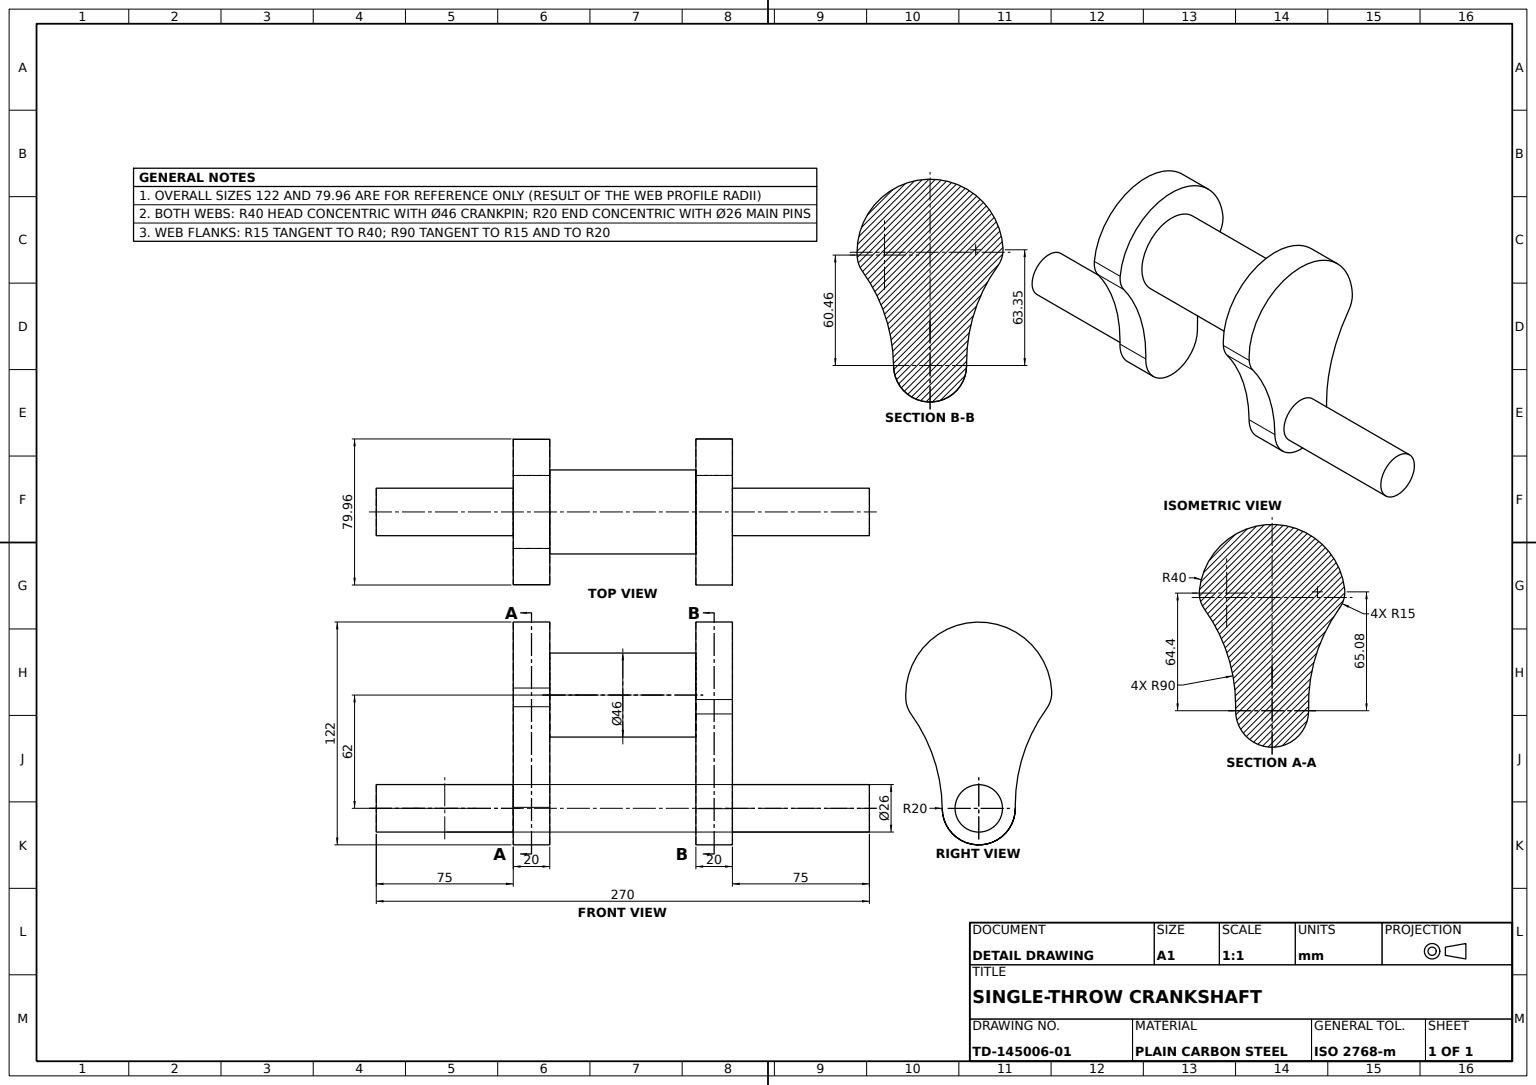
from build123d import *

# Parameters (mm, degrees)
FRONT_PLATE_DEPTH      = 20
FRONT_PIN_PROFILE_26_R = 13
FRONT_PIN_26_DEPTH     = 75
JOURNAL_PROFILE_46_R   = 23
JOURNAL_46_DEPTH       = 80
REAR_START             = -20
REAR_PLATE_DEPTH       = 20
REAR_START_2           = 75
REAR_PIN_PROFILE_26_R  = 13
REAR_PIN_26_DEPTH      = 75


with BuildPart() as part:
    # Front Plate Profile → Front Plate (new body)
    with BuildSketch(Plane.XY):
        with BuildLine():
            ThreePointArc((-19.989200766, 0.657155043), (-0.067809086, -19.999885048), (19.993197289, 0.52159577))
            ThreePointArc((19.993197289, 0.52159577), (23.983612751, 29.469835271), (37.03816485, 55.613718978))
            ThreePointArc((37.03816485, 55.613718978), (39.360775458, 60.47698398), (39.814551695, 65.847268297))
            ThreePointArc((39.814551695, 65.847268297), (0.541840926, 101.996329937), (-39.695719365, 66.9244151))
            ThreePointArc((-39.695719365, 66.9244151), (-39.339964644, 61.352839249), (-36.971364547, 56.297272766))
            ThreePointArc((-36.971364547, 56.297272766), (-23.860759515, 29.887158775), (-19.989200766, 0.657155043))
        make_face()
    extrude(amount=FRONT_PLATE_DEPTH)

    # Front Pin Profile Ø26 → Front Pin Ø26 (add)
    with BuildSketch(Plane.XY.offset(20)):
        Circle(FRONT_PIN_PROFILE_26_R)
    extrude(amount=FRONT_PIN_26_DEPTH)

    # Journal Profile Ø46 → Journal Ø46 (add)
    with BuildSketch(Plane(origin=(0, 0, 0), x_dir=(-1, 0, 0), z_dir=(0, 0, -1))):
        with Locations(Location((0, 62, 0), (0, 0, 180))):
            Circle(JOURNAL_PROFILE_46_R)
    extrude(amount=JOURNAL_46_DEPTH)

    # Rear Plate Profile → Rear Plate (add)
    with BuildSketch(Plane.XY.offset(-80).offset(REAR_START)):
        with BuildLine():
            ThreePointArc((-19.997507027, 0.315773186), (-0.260135851, -19.998308162), (19.998954502, -0.204496502))
            ThreePointArc((19.998954502, -0.204496502), (24.520770215, 27.058319007), (37.101446898, 51.663897663))
            ThreePointArc((37.101446898, 51.663897663), (39.072985568, 55.400775042), (39.924234273, 59.539203839))
            ThreePointArc((39.924234273, 59.539203839), (2.310034684, 101.933241038), (-39.941678501, 64.159240274))
            ThreePointArc((-39.941678501, 64.159240274), (-39.351963031, 59.110003561), (-37.109654718, 54.547700507))
            ThreePointArc((-37.109654718, 54.547700507), (-24.157614064, 28.818824435), (-19.997507027, 0.315773186))
        make_face()
    extrude(amount=REAR_PLATE_DEPTH)

    # Rear Pin Profile Ø26 → Rear Pin Ø26 (add)
    with BuildSketch(Plane(origin=(0, 0, -100), x_dir=(-1, 0, 0), z_dir=(0, 0, -1)).offset(REAR_START_2)):
        with Locations(Location((0, 0, 0), (0, 0, 180))):
            Circle(REAR_PIN_PROFILE_26_R)
    extrude(amount=-REAR_PIN_26_DEPTH)


solid = part.part
